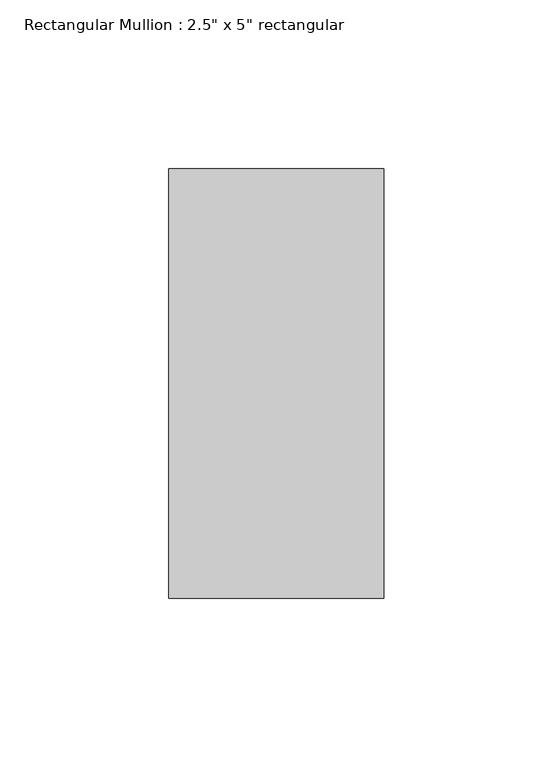
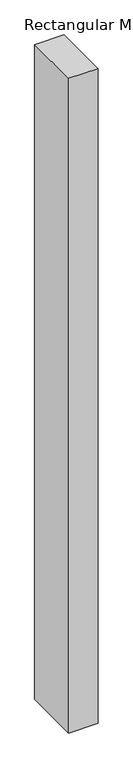
"""IFC4 building model written with IfcOpenShell, lengths in millimetres: member geometry."""

from ifc_helpers import new_model, si_unit, frame, origin, place, context, project, spatial, polyline, outline, extrude, source, transform, mapped, element, save


def member_0131f3aa(model_context):
    return source(origin(), model_context, "Body", "SweptSolid", [
        extrude(outline(polyline([(31.75, 63.5), (31.75, -63.5), (-31.75, -63.5), (-31.75, 63.5), (31.75, 63.5)])), frame((0.0, 0.0, -1492.25), z_axis=(0.0, 0.0, 1.0), x_axis=(1.0, 0.0, 0.0)), (0.0, 0.0, 1.0), 1492.25),
    ])


if __name__ == "__main__":
    model = new_model("IFC4")
    model_context = context("Model", 3, world=origin())
    ifc_project = project(units=[si_unit("LENGTHUNIT", "METRE", prefix="MILLI")], contexts=[model_context])
    site = spatial("IfcSite", under=ifc_project)
    building = spatial("IfcBuilding", under=site)
    placement = place(None, origin())
    member_shape = member_0131f3aa(model_context)
    element("IfcMember", 1, ObjectType="Rectangular Mullion : 2.5\" x 5\" rectangular", at=placement, inside=building, context=model_context, shape_type="MappedRepresentation", body=[
        mapped(member_shape, transform((0.0, 0.0, 0.0), x_axis=(1.0, 0.0, 0.0), y_axis=(0.0, 1.0, 0.0), z_axis=(0.0, 0.0, 1.0))),
    ])
    save(model, "model.ifc")

# Revit data of these elements
# Type "Rectangular Mullion : 2.5\" x 5\" rectangular"
#   built-in parameter 1007304 = 0.416667 (stored number, unit not read)
#   built-in parameter 1007301 = 0.104167 (stored number, unit not read)
#   built-in parameter 1007300 = 0.104167 (stored number, unit not read)
# Element 1 (IfcMember, "Rectangular Mullion : 2.5\" x 5\" rectangular")
#   Materials on its faces: "Aluminum"
# Materials
#   "Aluminum": class "Metal", colour RGB 247 247 247, transparency 0, Description = "Aluminum 6061", Cost = 0
